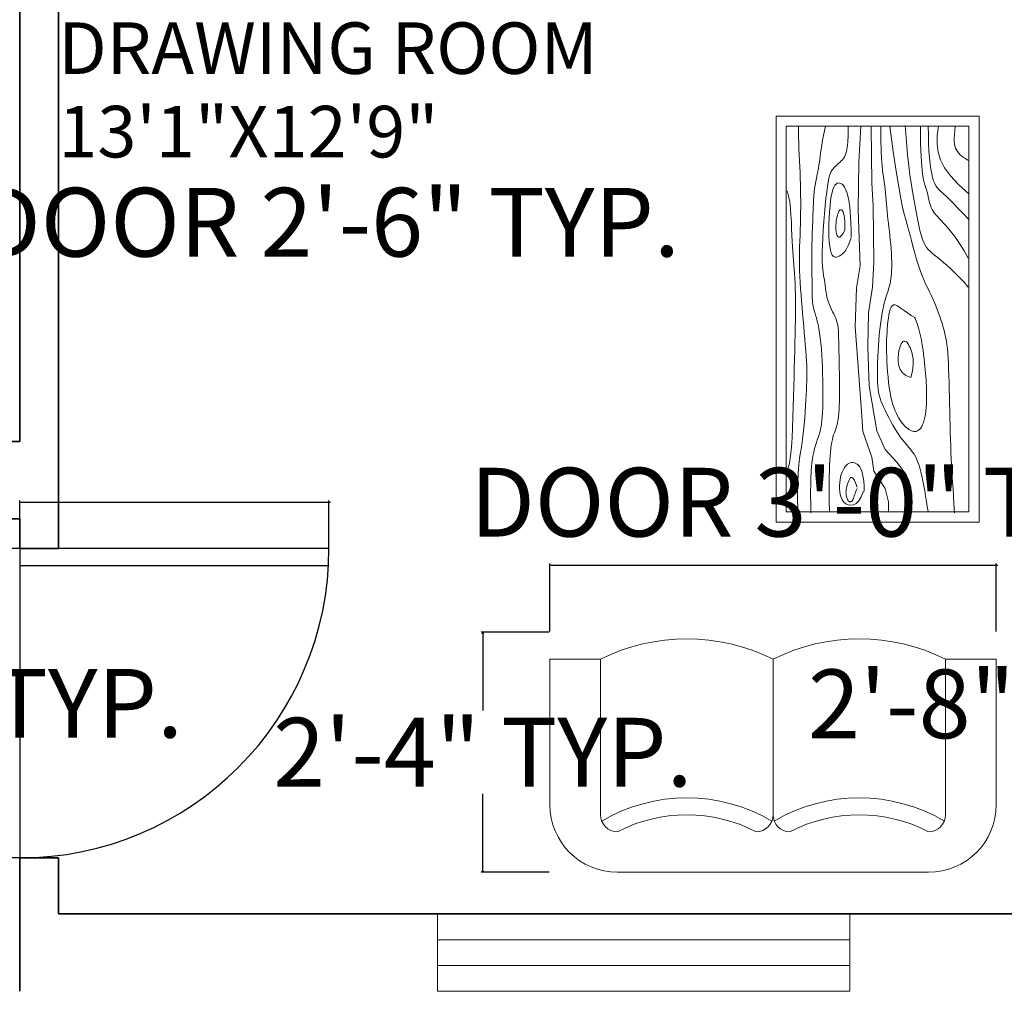
# Model space of a CAD drawing. Units: inches. Extents: x -11 to 443, y 65 to 743.
# Tile 3 of 10: x 162 to 276, y 212 to 325. Entities that reach past the tile are written whole.
import ezdxf

# ---------------------------------------------------------------- set-up
doc = ezdxf.new("R2010")
doc.units = ezdxf.units.IN
doc.header["$MEASUREMENT"] = 0
for name, color, linetype, lineweight in [('A-ANNO-DIMS', 2, 'Continuous', 18), ('A-AREA-IDEN', 2, 'Continuous', 18), ('A-DOOR', 4, 'Continuous', 25), ('A-GLAZ', 4, 'Continuous', 18), ('A-WALL', 7, 'Continuous', 35), ('Furniture', 7, 'Continuous', 15)]:
    doc.layers.add(name, color=color, linetype=linetype, lineweight=lineweight)
doc.styles.get("Standard").update_dxf_attribs({"font": 'italic8.shx'})
doc.dimstyles.get("Standard").update_dxf_attribs({"dimtxt": 8, "dimasz": 0.18, "dimexe": 0.18, "dimexo": 0.0625, "dimgap": 0.09, "dimtad": 0, "dimtih": 1, "dimtoh": 1, "dimzin": 0, "dimdsep": 46, "dimlunit": 3, "dimtxsty": 'Standard', "dimblk": 'CLOSEDBLANK', "dimcen": 0.09, "dimclrd": 6, "dimclre": 5, "dimclrt": 4, "dimadec": 0, "dimazin": 0, "dimtfac": 1, "dimtofl": 0, "dimtmove": 0, "dimatfit": 3, "dimfxl": 1, "dimtolj": 1, "dimtzin": 0, "dimarcsym": 0})

# ---------------------------------------------------------------- blocks, each defined once
blk = doc.blocks.new('DOOR-SWING-36')
for p, q in [((36, 36), (0, 36)), ((0, 36), (0, 0)), ((35.94, 34), (0, 34))]:
    blk.add_line(p, q)
blk.add_arc((0, 36), 36, 270, 0)
blk = doc.blocks.new('WIN-48x9')
for p, q in [((0, 48), (0, 0)), ((9, 48), (0, 48)), ((3, 0), (3, 48)), ((6, 0), (6, 48)), ((9, 0), (9, 48)), ((0, 0), (9, 0))]:
    blk.add_line(p, q)
blk = doc.blocks.new('LOVESEAT')
for p, q in [((0, 24.8, -27), (0, 7.87, -27)), ((0, 24.8, -27), (5.91, 24.8, -27)), ((5.91, 6.69, -27), (5.91, 24.8, -27)), ((25.98, 24.8, -27), (25.98, 6.69, -27)), ((25.98, 6.69, -27), (25.98, 24.8, -27)), ((46.06, 6.69, -27), (46.06, 24.8, -27)), ((46.06, 24.8, -27), (46.06, 6.69, -27)), ((46.06, 6.69, -27), (46.06, 24.8, -27)), ((51.97, 24.8, -27), (46.06, 24.8, -27)), ((51.97, 7.87, -27), (51.97, 24.8, -27)), ((7.87, 0, -27), (44.09, 0, -27))]:
    blk.add_line(p, q)
for centre, radius, start, end in [((15.94, 4.65, -27), 22.51, 63.519, 116.481), ((36.02, 4.65, -27), 22.51, 63.519, 116.481), ((15.94, -10.84, -27), 19.5, 59.4911, 120.5089), ((36.02, -10.84, -27), 19.5, 59.4911, 120.5089), ((7.87, 7.87, -27), 7.87, 180, 270), ((44.09, 7.87, -27), 7.87, 270, 0), ((7.87, 6.69, -27), 1.97, 180, 270), ((15.94, -10.84, -27), 17.53, 62.5861, 117.4139), ((24.02, 6.69, -27), 1.97, 270, 0), ((27.95, 6.69, -27), 1.97, 180, 270), ((36.02, -10.84, -27), 17.53, 62.5861, 117.4139), ((44.09, 6.69, -27), 1.97, 270, 0)]:
    blk.add_arc(centre, radius, start, end)
blk = doc.blocks.new('_ClosedBlank')
at = {"color": 0, "linetype": 'ByBlock', "lineweight": -2}
for p, q in [((-1, 0.167), (0, 0)), ((-1, 0.167), (-1, -0.167)), ((0, 0), (-1, -0.167))]:
    blk.add_line(p, q, dxfattribs=at)
blk = doc.blocks.new('*D20')
at = {"layer": 'A-ANNO-DIMS', "color": 5, "lineweight": -2, "transparency": 16777216}
for p, q in [((110.2, 296.98), (110.2, 301.6)), ((140.2, 296.98), (140.2, 301.6))]:
    blk.add_line(p, q, dxfattribs=at)
at = {"layer": 'A-ANNO-DIMS', "color": 6, "lineweight": -2, "transparency": 16777216}
for p, q in [((110.38, 301.42), (140.02, 301.42)), ((140.2, 301.42), (140.38, 301.42))]:
    blk.add_line(p, q, dxfattribs=at)
at = {"layer": 'Defpoints', "color": 0, "lineweight": 100, "transparency": 16777216}
for p in [(140.2, 301.42), (110.2, 296.92), (140.2, 296.92)]:
    blk.add_point(p, dxfattribs=at)
at = {"layer": 'A-ANNO-DIMS', "color": 6, "lineweight": -2, "transparency": 16777216, "xscale": 0.18, "yscale": 0.18, "zscale": 0.18, "rotation": 180}
blk.add_blockref('_ClosedBlank', (110.2, 301.42), dxfattribs=at)
at = {"layer": 'A-ANNO-DIMS', "color": 6, "lineweight": -2, "transparency": 16777216, "xscale": 0.18, "yscale": 0.18, "zscale": 0.18}
blk.add_blockref('_ClosedBlank', (140.2, 301.42), dxfattribs=at)
at = {"layer": 'A-ANNO-DIMS', "color": 4, "transparency": 16777216, "insert": (197.61, 301.42), "char_height": 8, "attachment_point": 5}
blk.add_mtext('\\A1;DOOR 2\'-6" TYP.', dxfattribs=at)
blk = doc.blocks.new('*D22')
at = {"layer": 'A-ANNO-DIMS', "color": 5, "lineweight": -2, "transparency": 16777216}
for p, q in [((161.71, 263.5), (161.71, 269.02)), ((197.71, 263.5), (197.71, 269.02))]:
    blk.add_line(p, q, dxfattribs=at)
at = {"layer": 'A-ANNO-DIMS', "color": 6, "lineweight": -2, "transparency": 16777216}
for p, q in [((161.89, 268.84), (197.53, 268.84)), ((197.71, 268.84), (197.89, 268.84))]:
    blk.add_line(p, q, dxfattribs=at)
at = {"layer": 'Defpoints', "color": 0, "lineweight": 100, "transparency": 16777216}
for p in [(197.71, 268.84), (161.71, 263.44), (197.71, 263.44)]:
    blk.add_point(p, dxfattribs=at)
at = {"layer": 'A-ANNO-DIMS', "color": 6, "lineweight": -2, "transparency": 16777216, "xscale": 0.18, "yscale": 0.18, "zscale": 0.18, "rotation": 180}
blk.add_blockref('_ClosedBlank', (161.71, 268.84), dxfattribs=at)
at = {"layer": 'A-ANNO-DIMS', "color": 6, "lineweight": -2, "transparency": 16777216, "xscale": 0.18, "yscale": 0.18, "zscale": 0.18}
blk.add_blockref('_ClosedBlank', (197.71, 268.84), dxfattribs=at)
at = {"layer": 'A-ANNO-DIMS', "color": 4, "transparency": 16777216, "insert": (255.12, 268.84), "char_height": 8, "attachment_point": 5}
blk.add_mtext('\\A1;DOOR 3\'-0" TYP.', dxfattribs=at)
blk = doc.blocks.new('*D23')
at = {"layer": 'A-ANNO-DIMS', "color": 5, "lineweight": -2, "transparency": 16777216}
for p, q in [((161.65, 263.44), (156.13, 263.44)), ((161.65, 227.44), (156.13, 227.44))]:
    blk.add_line(p, q, dxfattribs=at)
at = {"layer": 'A-ANNO-DIMS', "color": 6, "lineweight": -2, "transparency": 16777216}
for p, q in [((156.31, 263.26), (156.31, 250.29)), ((156.31, 227.62), (156.31, 240.59))]:
    blk.add_line(p, q, dxfattribs=at)
at = {"layer": 'Defpoints', "color": 0, "lineweight": 100, "transparency": 16777216}
for p in [(156.31, 263.44), (161.71, 263.44), (161.71, 227.44)]:
    blk.add_point(p, dxfattribs=at)
at = {"layer": 'A-ANNO-DIMS', "color": 6, "lineweight": -2, "transparency": 16777216, "xscale": 0.18, "yscale": 0.18, "zscale": 0.18}
for p, rotation in [((156.31, 263.44), 90), ((156.31, 227.44), 270)]:
    blk.add_blockref('_ClosedBlank', p, dxfattribs=dict(at, rotation=rotation))
at = {"layer": 'A-ANNO-DIMS', "color": 4, "transparency": 16777216, "insert": (156.31, 245.44), "char_height": 8, "attachment_point": 5}
blk.add_mtext('\\A1;3\'-0" TYP.', dxfattribs=at)
blk = doc.blocks.new('*D32')
at = {"layer": 'A-ANNO-DIMS', "color": 5, "lineweight": -2, "transparency": 16777216}
for p, q in [((223.42, 253.79), (223.42, 261.7)), ((275.39, 253.79), (275.39, 261.7))]:
    blk.add_line(p, q, dxfattribs=at)
at = {"layer": 'A-ANNO-DIMS', "color": 6, "lineweight": -2, "transparency": 16777216}
for p, q in [((223.6, 261.52), (275.21, 261.52)), ((275.39, 261.52), (275.57, 261.52))]:
    blk.add_line(p, q, dxfattribs=at)
at = {"layer": 'Defpoints', "color": 0, "lineweight": 100, "transparency": 16777216}
for p in [(275.39, 261.52), (223.42, 253.72), (275.39, 253.72)]:
    blk.add_point(p, dxfattribs=at)
at = {"layer": 'A-ANNO-DIMS', "color": 6, "lineweight": -2, "transparency": 16777216, "xscale": 0.18, "yscale": 0.18, "zscale": 0.18, "rotation": 180}
blk.add_blockref('_ClosedBlank', (223.42, 261.52), dxfattribs=at)
at = {"layer": 'A-ANNO-DIMS', "color": 6, "lineweight": -2, "transparency": 16777216, "xscale": 0.18, "yscale": 0.18, "zscale": 0.18}
blk.add_blockref('_ClosedBlank', (275.39, 261.52), dxfattribs=at)
at = {"layer": 'A-ANNO-DIMS', "color": 4, "transparency": 16777216, "insert": (349.75, 261.52), "char_height": 8, "attachment_point": 5}
blk.add_mtext('\\A1;LOVESEAT 4\'-4" TYP.', dxfattribs=at)
blk = doc.blocks.new('*D33')
at = {"layer": 'A-ANNO-DIMS', "color": 5, "lineweight": -2, "transparency": 16777216}
for p, q in [((223.36, 253.72), (215.44, 253.72)), ((223.36, 225.77), (215.44, 225.77))]:
    blk.add_line(p, q, dxfattribs=at)
at = {"layer": 'A-ANNO-DIMS', "color": 6, "lineweight": -2, "transparency": 16777216}
for p, q in [((215.62, 253.54), (215.62, 244.6)), ((215.62, 225.95), (215.62, 234.89))]:
    blk.add_line(p, q, dxfattribs=at)
at = {"layer": 'Defpoints', "color": 0, "lineweight": 100, "transparency": 16777216}
for p in [(215.62, 253.72), (223.42, 253.72), (223.42, 225.77)]:
    blk.add_point(p, dxfattribs=at)
at = {"layer": 'A-ANNO-DIMS', "color": 6, "lineweight": -2, "transparency": 16777216, "xscale": 0.18, "yscale": 0.18, "zscale": 0.18}
for p, rotation in [((215.62, 253.72), 90), ((215.62, 225.77), 270)]:
    blk.add_blockref('_ClosedBlank', p, dxfattribs=dict(at, rotation=rotation))
at = {"layer": 'A-ANNO-DIMS', "color": 4, "transparency": 16777216, "insert": (215.62, 239.75), "char_height": 8, "attachment_point": 5}
blk.add_mtext('\\A1;2\'-4" TYP.', dxfattribs=at)
blk = doc.blocks.new('*D35')
at = {"layer": 'A-ANNO-DIMS', "color": 5, "lineweight": -2, "transparency": 16777216}
for p, q in [((282.97, 261.39), (277.7, 261.39)), ((282.97, 229.35), (277.7, 229.35))]:
    blk.add_line(p, q, dxfattribs=at)
at = {"layer": 'A-ANNO-DIMS', "color": 6, "lineweight": -2, "transparency": 16777216}
for p, q in [((277.88, 261.21), (277.88, 250.22)), ((277.88, 229.53), (277.88, 240.52))]:
    blk.add_line(p, q, dxfattribs=at)
at = {"layer": 'Defpoints', "color": 0, "lineweight": 100, "transparency": 16777216}
for p in [(277.88, 261.39), (283.03, 261.39), (283.03, 229.35)]:
    blk.add_point(p, dxfattribs=at)
at = {"layer": 'A-ANNO-DIMS', "color": 6, "lineweight": -2, "transparency": 16777216, "xscale": 0.18, "yscale": 0.18, "zscale": 0.18}
for p, rotation in [((277.88, 261.39), 90), ((277.88, 229.35), 270)]:
    blk.add_blockref('_ClosedBlank', p, dxfattribs=dict(at, rotation=rotation))
at = {"layer": 'A-ANNO-DIMS', "color": 4, "transparency": 16777216, "insert": (277.88, 245.37), "char_height": 8, "attachment_point": 5}
blk.add_mtext('\\A1;2\'-8" TYP.', dxfattribs=at)

msp = doc.modelspace()

# ---------------------------------------------------------------- linework, layer by layer
at = {"layer": 'A-WALL'}
for p, q in [((161.709, 275.92), (161.709, 373.92)), ((166.209, 263.442), (166.209, 373.92)), ((140.201, 275.92), (161.709, 275.92)), ((140.201, 266.92), (161.709, 266.92)), ((161.709, 263.442), (161.709, 266.92)), ((161.709, 263.442), (166.209, 263.442)), ((161.709, 211.92), (161.709, 227.442)), ((161.709, 227.442), (166.209, 227.442)), ((166.209, 220.92), (166.209, 227.442)), ((166.209, 220.92), (323.209, 220.92))]:
    msp.add_line(p, q, dxfattribs=at)
at = {"layer": 'Furniture'}
for p, q in [((249.755, 266.524), (249.755, 313.768)), ((249.755, 313.768), (273.377, 313.768)), ((273.377, 313.768), (273.377, 266.524)), ((250.936, 267.705), (250.936, 312.587)), ((250.936, 312.587), (272.196, 312.587)), ((252.347, 312.524), (252.353, 311.905)), ((252.353, 311.905), (252.367, 311.265)), ((255.496, 312.605), (255.31, 311.718)), ((258.161, 312.524), (258.146, 311.54)), ((259.614, 312.605), (259.372, 308.404)), ((260.826, 312.524), (260.906, 305.98)), ((261.956, 312.524), (261.967, 311.013)), ((263.006, 312.605), (263.399, 309.671)), ((264.782, 312.685), (264.93, 310.824)), ((266.559, 312.524), (266.578, 310.594)), ((267.474, 312.632), (267.483, 311.568)), ((268.658, 312.605), (268.522, 311.512)), ((270.543, 312.067), (270.507, 311.601)), ((270.596, 312.605), (270.543, 312.067)), ((272.196, 312.587), (272.196, 267.705)), ((252.367, 311.265), (252.39, 310.606)), ((252.39, 310.606), (252.417, 309.934)), ((255.168, 310.983), (255.062, 310.374)), ((255.31, 311.718), (255.168, 310.983)), ((258.105, 310.754), (258.04, 310.138)), ((258.146, 311.54), (258.105, 310.754)), ((261.967, 311.013), (261.996, 309.787)), ((264.93, 310.824), (265.071, 309.271)), ((267.483, 311.568), (267.51, 310.597)), ((267.51, 310.597), (267.554, 309.716)), ((268.522, 311.512), (268.498, 310.516)), ((270.507, 311.601), (270.49, 311.198)), ((270.49, 311.198), (270.492, 310.85)), ((270.492, 310.85), (270.517, 310.548)), ((252.417, 309.934), (252.448, 309.253)), ((254.985, 309.868), (254.928, 309.442)), ((255.062, 310.374), (254.985, 309.868)), ((257.954, 309.667), (257.851, 309.313)), ((258.04, 310.138), (257.954, 309.667)), ((261.996, 309.787), (262.04, 308.803)), ((263.399, 309.671), (263.735, 307.353)), ((266.578, 310.594), (266.632, 309.07)), ((267.554, 309.716), (267.612, 308.925)), ((268.498, 310.516), (268.611, 309.581)), ((268.611, 309.581), (268.89, 308.676)), ((270.517, 310.548), (270.565, 310.284)), ((270.565, 310.284), (270.638, 310.05)), ((270.638, 310.05), (270.737, 309.838)), ((270.737, 309.838), (270.864, 309.64)), ((270.864, 309.64), (271.016, 309.454)), ((271.016, 309.454), (271.187, 309.281)), ((252.448, 309.253), (252.481, 308.567)), ((252.481, 308.567), (252.513, 307.881)), ((254.797, 308.404), (254.74, 308.063)), ((254.842, 308.733), (254.797, 308.404)), ((254.883, 309.071), (254.842, 308.733)), ((254.928, 309.442), (254.883, 309.071)), ((257.197, 308.416), (257.056, 308.288)), ((257.337, 308.55), (257.197, 308.416)), ((257.475, 308.693), (257.337, 308.55)), ((257.608, 308.853), (257.475, 308.693)), ((257.735, 309.05), (257.608, 308.853)), ((257.851, 309.313), (257.735, 309.05)), ((259.372, 308.404), (259.291, 302.829)), ((262.04, 308.803), (262.096, 308.02)), ((265.071, 309.271), (265.206, 307.98)), ((266.632, 309.07), (266.712, 307.892)), ((267.612, 308.925), (267.686, 308.22)), ((268.89, 308.676), (269.362, 307.768)), ((271.187, 309.281), (271.376, 309.118)), ((271.376, 309.118), (271.576, 308.966)), ((271.576, 308.966), (271.785, 308.824)), ((271.785, 308.824), (271.998, 308.69)), ((271.998, 308.69), (272.211, 308.565)), ((252.513, 307.881), (252.542, 307.199)), ((252.542, 307.199), (252.568, 306.523)), ((254.602, 307.34), (254.526, 306.96)), ((254.674, 307.708), (254.602, 307.34)), ((254.74, 308.063), (254.674, 307.708)), ((256.182, 307.327), (256.084, 307.114)), ((256.286, 307.501), (256.182, 307.327)), ((256.398, 307.65), (256.286, 307.501)), ((256.518, 307.786), (256.398, 307.65)), ((256.646, 307.916), (256.518, 307.786)), ((256.779, 308.041), (256.646, 307.916)), ((256.916, 308.164), (256.779, 308.041)), ((257.056, 308.288), (256.916, 308.164)), ((262.096, 308.02), (262.158, 307.396)), ((262.158, 307.396), (262.223, 306.889)), ((263.735, 307.353), (264.024, 305.557)), ((265.206, 307.98), (265.336, 306.908)), ((266.712, 307.892), (266.812, 307.005)), ((267.686, 308.22), (267.772, 307.6)), ((267.772, 307.6), (267.87, 307.063)), ((269.362, 307.768), (270.055, 306.822)), ((252.568, 306.523), (252.589, 305.855)), ((254.375, 306.166), (254.306, 305.754)), ((254.449, 306.568), (254.375, 306.166)), ((254.526, 306.96), (254.449, 306.568)), ((255.815, 306.091), (255.73, 305.574)), ((255.902, 306.511), (255.815, 306.091)), ((255.991, 306.847), (255.902, 306.511)), ((256.084, 307.114), (255.991, 306.847)), ((262.223, 306.889), (262.287, 306.458)), ((262.287, 306.458), (262.346, 306.061)), ((262.346, 306.061), (262.398, 305.663)), ((265.336, 306.908), (265.461, 306.01)), ((266.812, 307.005), (266.923, 306.351)), ((266.923, 306.351), (267.038, 305.872)), ((267.87, 307.063), (267.978, 306.606)), ((267.978, 306.606), (268.097, 306.227)), ((268.097, 306.227), (268.224, 305.916)), ((270.055, 306.822), (270.995, 305.806)), ((251.055, 305.091), (251.215, 304.472)), ((252.589, 305.855), (252.605, 305.191)), ((252.605, 305.191), (252.616, 304.532)), ((254.195, 304.906), (254.154, 304.474)), ((254.245, 305.334), (254.195, 304.906)), ((254.306, 305.754), (254.245, 305.334)), ((255.644, 304.943), (255.558, 304.193)), ((255.73, 305.574), (255.644, 304.943)), ((256.275, 304.886), (256.183, 304.453)), ((256.377, 305.237), (256.275, 304.886)), ((256.487, 305.514), (256.377, 305.237)), ((256.606, 305.722), (256.487, 305.514)), ((256.732, 305.867), (256.606, 305.722)), ((256.865, 305.955), (256.732, 305.867)), ((257.004, 305.994), (256.865, 305.955)), ((257.147, 305.986), (257.004, 305.994)), ((257.293, 305.934), (257.147, 305.986)), ((257.439, 305.835), (257.293, 305.934)), ((257.583, 305.688), (257.439, 305.835)), ((257.722, 305.492), (257.583, 305.688)), ((257.854, 305.247), (257.722, 305.492)), ((257.977, 304.95), (257.854, 305.247)), ((258.087, 304.6), (257.977, 304.95)), ((260.906, 305.98), (261.068, 303.314)), ((262.398, 305.663), (262.442, 305.258)), ((262.442, 305.258), (262.482, 304.846)), ((264.024, 305.557), (264.272, 304.19)), ((265.461, 306.01), (265.583, 305.241)), ((265.583, 305.241), (265.702, 304.557)), ((267.038, 305.872), (267.15, 305.512)), ((267.15, 305.512), (267.252, 305.213)), ((267.252, 305.213), (267.337, 304.927)), ((267.337, 304.927), (267.408, 304.646)), ((268.224, 305.916), (268.36, 305.66)), ((268.36, 305.66), (268.504, 305.449)), ((268.504, 305.449), (268.656, 305.271)), ((268.656, 305.271), (268.816, 305.115)), ((268.816, 305.115), (268.982, 304.969)), ((268.982, 304.969), (269.156, 304.822)), ((270.995, 305.806), (272.211, 304.688)), ((251.215, 304.472), (251.337, 303.779)), ((251.337, 303.779), (251.426, 303.032)), ((252.616, 304.532), (252.621, 303.874)), ((252.621, 303.874), (252.621, 303.218)), ((254.122, 304.038), (254.097, 303.602)), ((254.154, 304.474), (254.122, 304.038)), ((255.558, 304.193), (255.474, 303.347)), ((256.102, 303.933), (256.032, 303.326)), ((256.183, 304.453), (256.102, 303.933)), ((258.183, 304.197), (258.087, 304.6)), ((258.265, 303.737), (258.183, 304.197)), ((258.334, 303.22), (258.265, 303.737)), ((262.482, 304.846), (262.518, 304.427)), ((262.518, 304.427), (262.553, 304)), ((262.553, 304), (262.589, 303.567)), ((264.272, 304.19), (264.487, 303.159)), ((265.702, 304.557), (265.818, 303.913)), ((265.818, 303.913), (265.934, 303.274)), ((267.408, 304.646), (267.47, 304.371)), ((267.47, 304.371), (267.528, 304.103)), ((267.528, 304.103), (267.587, 303.844)), ((267.587, 303.844), (267.65, 303.594)), ((269.156, 304.822), (269.338, 304.661)), ((269.338, 304.661), (269.544, 304.471)), ((269.544, 304.471), (269.789, 304.233)), ((269.789, 304.233), (270.089, 303.93)), ((270.089, 303.93), (270.463, 303.545)), ((251.426, 303.032), (251.489, 302.253)), ((252.621, 303.218), (252.615, 302.56)), ((254.059, 302.738), (254.044, 302.315)), ((254.076, 303.168), (254.059, 302.738)), ((254.097, 303.602), (254.076, 303.168)), ((255.474, 303.347), (255.393, 302.435)), ((255.975, 302.65), (255.933, 301.932)), ((256.032, 303.326), (255.975, 302.65)), ((257.059, 302.692), (257.002, 302.568)), ((257.12, 302.786), (257.059, 302.692)), ((257.183, 302.848), (257.12, 302.786)), ((257.25, 302.877), (257.183, 302.848)), ((257.32, 302.871), (257.25, 302.877)), ((257.394, 302.829), (257.32, 302.871)), ((257.471, 302.749), (257.394, 302.829)), ((257.547, 302.622), (257.471, 302.749)), ((257.619, 302.443), (257.547, 302.622)), ((258.389, 302.642), (258.334, 303.22)), ((258.431, 302.001), (258.389, 302.642)), ((259.291, 302.829), (259.534, 296.366)), ((261.068, 303.314), (261.149, 296.77)), ((262.589, 303.567), (262.627, 303.127)), ((262.627, 303.127), (262.669, 302.681)), ((262.669, 302.681), (262.718, 302.229)), ((264.487, 303.159), (264.678, 302.372)), ((265.934, 303.274), (266.049, 302.639)), ((266.049, 302.639), (266.166, 302.017)), ((267.65, 303.594), (267.723, 303.354)), ((267.723, 303.354), (267.81, 303.126)), ((267.81, 303.126), (267.915, 302.909)), ((267.915, 302.909), (268.04, 302.7)), ((268.04, 302.7), (268.184, 302.495)), ((270.463, 303.545), (270.925, 303.061)), ((270.925, 303.061), (271.493, 302.46)), ((251.489, 302.253), (251.534, 301.462)), ((251.534, 301.462), (251.566, 300.681)), ((252.603, 301.9), (252.585, 301.237)), ((252.615, 302.56), (252.603, 301.9)), ((254.014, 301.496), (253.998, 301.095)), ((254.029, 301.9), (254.014, 301.496)), ((254.044, 302.315), (254.029, 301.9)), ((255.318, 301.49), (255.252, 300.542)), ((255.393, 302.435), (255.318, 301.49)), ((255.933, 301.932), (255.907, 301.199)), ((256.765, 301.57), (256.735, 301.32)), ((256.803, 301.809), (256.765, 301.57)), ((256.847, 302.033), (256.803, 301.809)), ((256.896, 302.237), (256.847, 302.033)), ((256.948, 302.416), (256.896, 302.237)), ((257.002, 302.568), (256.948, 302.416)), ((257.682, 302.203), (257.619, 302.443)), ((257.731, 301.895), (257.682, 302.203)), ((257.763, 301.512), (257.731, 301.895)), ((257.773, 301.045), (257.763, 301.512)), ((258.461, 301.295), (258.431, 302.001)), ((262.718, 302.229), (262.771, 301.769)), ((262.771, 301.769), (262.827, 301.303)), ((264.678, 302.372), (264.852, 301.734)), ((264.852, 301.734), (265.018, 301.153)), ((266.166, 302.017), (266.284, 301.418)), ((268.184, 302.495), (268.347, 302.289)), ((268.347, 302.289), (268.529, 302.077)), ((268.529, 302.077), (268.732, 301.855)), ((268.732, 301.855), (268.954, 301.618)), ((268.954, 301.618), (269.196, 301.362)), ((271.493, 302.46), (272.184, 301.725)), ((251.566, 300.681), (251.593, 299.929)), ((252.563, 300.57), (252.54, 299.899)), ((252.585, 301.237), (252.563, 300.57)), ((253.981, 300.691), (253.966, 300.276)), ((253.998, 301.095), (253.981, 300.691)), ((255.252, 300.542), (255.198, 299.623)), ((255.907, 301.199), (255.898, 300.474)), ((255.898, 300.474), (255.909, 299.785)), ((256.716, 301.064), (256.71, 300.807)), ((256.71, 300.807), (256.717, 300.555)), ((256.735, 301.32), (256.716, 301.064)), ((256.717, 300.555), (256.741, 300.312)), ((256.741, 300.312), (256.783, 300.084)), ((257.532, 300.082), (257.757, 300.487)), ((257.757, 300.487), (257.773, 301.045)), ((258.478, 300.522), (258.461, 301.295)), ((258.484, 299.679), (258.478, 300.522)), ((262.827, 301.303), (262.885, 300.828)), ((262.885, 300.828), (262.942, 300.346)), ((262.942, 300.346), (262.999, 299.854)), ((265.018, 301.153), (265.182, 300.554)), ((265.182, 300.554), (265.346, 299.928)), ((266.284, 301.418), (266.406, 300.85)), ((266.406, 300.85), (266.532, 300.322)), ((266.532, 300.322), (266.663, 299.844)), ((269.196, 301.362), (269.459, 301.08)), ((269.459, 301.08), (269.745, 300.76)), ((269.745, 300.76), (270.058, 300.388)), ((270.058, 300.388), (270.401, 299.95)), ((251.593, 299.929), (251.621, 299.228)), ((251.621, 299.228), (251.654, 298.592)), ((252.517, 299.224), (252.498, 298.546)), ((252.54, 299.899), (252.517, 299.224)), ((253.939, 299.384), (253.929, 298.892)), ((253.951, 299.843), (253.939, 299.384)), ((253.966, 300.276), (253.951, 299.843)), ((255.198, 299.623), (255.157, 298.764)), ((255.909, 299.785), (255.94, 299.157)), ((255.94, 299.157), (255.994, 298.615)), ((256.783, 300.084), (256.846, 299.89)), ((256.846, 299.89), (256.931, 299.748)), ((256.931, 299.748), (257.04, 299.677)), ((257.04, 299.677), (257.175, 299.696)), ((257.175, 299.696), (257.338, 299.825)), ((257.338, 299.825), (257.532, 300.082)), ((258.201, 298.792), (258.352, 299.17)), ((258.352, 299.17), (258.484, 299.598)), ((262.999, 299.854), (263.052, 299.354)), ((263.052, 299.354), (263.1, 298.844)), ((265.346, 299.928), (265.511, 299.285)), ((265.511, 299.285), (265.68, 298.636)), ((266.663, 299.844), (266.801, 299.423)), ((266.801, 299.423), (266.947, 299.065)), ((270.401, 299.95), (270.776, 299.431)), ((270.776, 299.431), (271.187, 298.819)), ((251.654, 298.592), (251.694, 298.013)), ((251.694, 298.013), (251.737, 297.477)), ((252.498, 298.546), (252.484, 297.864)), ((253.922, 298.359), (253.919, 297.782)), ((253.929, 298.892), (253.922, 298.359)), ((255.133, 297.996), (255.127, 297.342)), ((255.157, 298.764), (255.133, 297.996)), ((255.994, 298.615), (256.072, 298.18)), ((256.072, 298.18), (256.171, 297.847)), ((257.67, 297.943), (257.857, 298.181)), ((257.857, 298.181), (258.035, 298.463)), ((258.035, 298.463), (258.201, 298.792)), ((263.1, 298.844), (263.142, 298.325)), ((263.142, 298.325), (263.176, 297.802)), ((265.68, 298.636), (265.851, 297.99)), ((265.851, 297.99), (266.027, 297.356)), ((266.947, 299.065), (267.104, 298.762)), ((267.104, 298.762), (267.277, 298.5)), ((267.277, 298.5), (267.469, 298.266)), ((267.469, 298.266), (267.684, 298.047)), ((267.684, 298.047), (267.927, 297.831)), ((271.187, 298.819), (271.637, 298.098)), ((271.637, 298.098), (272.13, 297.255)), ((251.737, 297.477), (251.782, 296.968)), ((251.782, 296.968), (251.827, 296.473)), ((252.484, 297.864), (252.478, 297.178)), ((252.478, 297.178), (252.482, 296.488)), ((253.919, 297.782), (253.918, 297.173)), ((253.918, 297.173), (253.921, 296.545)), ((255.127, 297.342), (255.137, 296.793)), ((256.171, 297.847), (256.289, 297.608)), ((256.289, 297.608), (256.425, 297.452)), ((256.425, 297.452), (256.576, 297.37)), ((256.576, 297.37), (256.74, 297.352)), ((256.74, 297.352), (256.915, 297.389)), ((256.915, 297.389), (257.098, 297.471)), ((257.098, 297.471), (257.287, 297.59)), ((257.287, 297.59), (257.479, 297.746)), ((257.479, 297.746), (257.67, 297.943)), ((263.176, 297.802), (263.201, 297.28)), ((263.201, 297.28), (263.214, 296.765)), ((266.027, 297.356), (266.209, 296.744)), ((267.927, 297.831), (268.201, 297.605)), ((268.201, 297.605), (268.51, 297.356)), ((268.51, 297.356), (268.857, 297.073)), ((268.857, 297.073), (269.24, 296.751)), ((251.827, 296.473), (251.87, 295.978)), ((251.87, 295.978), (251.91, 295.467)), ((252.482, 296.488), (252.498, 295.794)), ((252.498, 295.794), (252.525, 295.096)), ((253.921, 296.545), (253.925, 295.915)), ((253.925, 295.915), (253.931, 295.298)), ((255.137, 296.793), (255.16, 296.331)), ((255.16, 296.331), (255.194, 295.939)), ((255.194, 295.939), (255.235, 295.598)), ((259.534, 296.366), (259.13, 293.781)), ((261.149, 296.77), (260.987, 293.862)), ((263.202, 295.782), (263.173, 295.325)), ((263.215, 296.264), (263.202, 295.782)), ((263.214, 296.765), (263.215, 296.264)), ((266.209, 296.744), (266.397, 296.165)), ((266.397, 296.165), (266.592, 295.624)), ((269.24, 296.751), (269.657, 296.387)), ((269.657, 296.387), (270.103, 295.98)), ((270.103, 295.98), (270.577, 295.527)), ((251.91, 295.467), (251.944, 294.926)), ((251.944, 294.926), (251.97, 294.344)), ((252.525, 295.096), (252.563, 294.393)), ((253.931, 295.298), (253.937, 294.709)), ((253.937, 294.709), (253.943, 294.162)), ((255.235, 295.598), (255.281, 295.292)), ((255.281, 295.292), (255.328, 295.002)), ((255.328, 295.002), (255.375, 294.71)), ((255.375, 294.71), (255.419, 294.404)), ((263.127, 294.899), (263.062, 294.507)), ((263.173, 295.325), (263.127, 294.899)), ((266.592, 295.624), (266.793, 295.119)), ((266.793, 295.119), (266.997, 294.644)), ((266.997, 294.644), (267.203, 294.194)), ((270.577, 295.527), (271.074, 295.024)), ((271.074, 295.024), (271.593, 294.47)), ((251.97, 294.344), (251.99, 293.719)), ((251.99, 293.719), (252.002, 293.053)), ((252.563, 294.393), (252.608, 293.685)), ((252.608, 293.685), (252.66, 292.972)), ((253.943, 294.162), (253.949, 293.674)), ((253.949, 293.674), (253.954, 293.254)), ((255.419, 294.404), (255.462, 294.083)), ((255.462, 294.083), (255.507, 293.752)), ((255.507, 293.752), (255.555, 293.416)), ((255.555, 293.416), (255.611, 293.08)), ((259.13, 293.781), (258.968, 289.257)), ((260.987, 293.862), (260.503, 290.873)), ((262.787, 293.456), (262.678, 293.118)), ((262.889, 293.795), (262.787, 293.456)), ((262.982, 294.142), (262.889, 293.795)), ((263.062, 294.507), (262.982, 294.142)), ((267.203, 294.194), (267.408, 293.761)), ((267.408, 293.761), (267.61, 293.341)), ((271.593, 294.47), (272.13, 293.862)), ((252.002, 293.053), (252.009, 292.349)), ((252.009, 292.349), (252.01, 291.607)), ((252.66, 292.972), (252.718, 292.252)), ((253.954, 293.254), (253.959, 292.896)), ((253.959, 292.896), (253.967, 292.589)), ((253.967, 292.589), (253.981, 292.32)), ((253.981, 292.32), (254.001, 292.08)), ((255.611, 293.08), (255.676, 292.747)), ((255.676, 292.747), (255.754, 292.423)), ((255.754, 292.423), (255.846, 292.112)), ((262.455, 292.401), (262.346, 292.004)), ((262.567, 292.769), (262.455, 292.401)), ((262.678, 293.118), (262.567, 292.769)), ((267.61, 293.341), (267.808, 292.928)), ((267.808, 292.928), (267.999, 292.516)), ((267.999, 292.516), (268.181, 292.1)), ((252.01, 291.607), (252.006, 290.83)), ((252.718, 292.252), (252.78, 291.526)), ((252.78, 291.526), (252.845, 290.792)), ((254.001, 292.08), (254.03, 291.856)), ((254.03, 291.856), (254.07, 291.637)), ((254.07, 291.637), (254.124, 291.412)), ((254.124, 291.412), (254.191, 291.17)), ((254.191, 291.17), (254.271, 290.905)), ((255.846, 292.112), (255.955, 291.817)), ((255.955, 291.817), (256.077, 291.537)), ((256.077, 291.537), (256.207, 291.268)), ((256.207, 291.268), (256.339, 291.008)), ((262.244, 291.571), (262.147, 291.104)), ((262.346, 292.004), (262.244, 291.571)), ((262.965, 290.992), (263.052, 291.294)), ((263.052, 291.294), (263.158, 291.538)), ((263.158, 291.538), (263.283, 291.711)), ((263.283, 291.711), (263.43, 291.802)), ((263.43, 291.802), (263.602, 291.802)), ((263.602, 291.802), (263.805, 291.722)), ((263.805, 291.722), (264.044, 291.574)), ((264.044, 291.574), (264.325, 291.373)), ((264.325, 291.373), (264.655, 291.132)), ((264.655, 291.132), (265.039, 290.865)), ((268.181, 292.1), (268.354, 291.682)), ((268.354, 291.682), (268.518, 291.265)), ((268.518, 291.265), (268.671, 290.853)), ((251.997, 290.019), (251.984, 289.176)), ((252.006, 290.83), (251.997, 290.019)), ((252.845, 290.792), (252.911, 290.053)), ((252.911, 290.053), (252.977, 289.313)), ((254.271, 290.905), (254.359, 290.611)), ((254.359, 290.611), (254.453, 290.284)), ((254.453, 290.284), (254.55, 289.918)), ((256.339, 291.008), (256.47, 290.752)), ((256.47, 290.752), (256.594, 290.499)), ((256.594, 290.499), (256.706, 290.244)), ((256.706, 290.244), (256.802, 289.984)), ((256.802, 289.984), (256.877, 289.717)), ((260.503, 290.873), (260.422, 286.914)), ((261.975, 290.072), (261.899, 289.513)), ((262.057, 290.603), (261.975, 290.072)), ((262.147, 291.104), (262.057, 290.603)), ((262.78, 289.859), (262.831, 290.263)), ((262.831, 290.263), (262.891, 290.645)), ((262.891, 290.645), (262.965, 290.992)), ((265.039, 290.865), (265.483, 290.585)), ((265.483, 290.585), (265.993, 290.307)), ((265.913, 290.307), (266.161, 289.644)), ((268.671, 290.853), (268.815, 290.448)), ((268.815, 290.448), (268.949, 290.054)), ((268.949, 290.054), (269.071, 289.674)), ((251.984, 289.176), (251.967, 288.303)), ((252.977, 289.313), (253.041, 288.581)), ((254.55, 289.918), (254.646, 289.507)), ((254.646, 289.507), (254.738, 289.046)), ((254.738, 289.046), (254.823, 288.53)), ((256.877, 289.717), (256.934, 289.435)), ((256.934, 289.435), (256.976, 289.131)), ((256.976, 289.131), (257.005, 288.798)), ((258.968, 289.257), (259.372, 283.602)), ((261.83, 288.929), (261.768, 288.322)), ((261.899, 289.513), (261.83, 288.929)), ((262.667, 288.616), (262.699, 289.032)), ((262.699, 289.032), (262.737, 289.446)), ((262.737, 289.446), (262.78, 289.859)), ((266.161, 289.644), (266.366, 288.989)), ((266.366, 288.989), (266.533, 288.347)), ((269.071, 289.674), (269.183, 289.311)), ((269.183, 289.311), (269.283, 288.966)), ((269.283, 288.966), (269.373, 288.63)), ((251.967, 288.303), (251.947, 287.396)), ((253.041, 288.581), (253.103, 287.864)), ((253.103, 287.864), (253.159, 287.169)), ((254.823, 288.53), (254.899, 287.956)), ((254.899, 287.956), (254.965, 287.331)), ((257.005, 288.798), (257.025, 288.429)), ((257.025, 288.429), (257.038, 288.017)), ((257.038, 288.017), (257.048, 287.555)), ((261.714, 287.695), (261.667, 287.052)), ((261.768, 288.322), (261.714, 287.695)), ((262.611, 287.302), (262.622, 287.756)), ((262.622, 287.756), (262.641, 288.192)), ((262.641, 288.192), (262.667, 288.616)), ((266.533, 288.347), (266.667, 287.723)), ((266.667, 287.723), (266.773, 287.123)), ((269.373, 288.63), (269.453, 288.292)), ((269.453, 288.292), (269.524, 287.941)), ((269.524, 287.941), (269.587, 287.566)), ((251.947, 287.396), (251.924, 286.454)), ((253.159, 287.169), (253.21, 286.505)), ((254.965, 287.331), (255.022, 286.666)), ((255.022, 286.666), (255.071, 285.969)), ((257.048, 287.555), (257.057, 287.036)), ((257.057, 287.036), (257.069, 286.455)), ((260.422, 286.914), (260.583, 282.39)), ((261.667, 287.052), (261.628, 286.4)), ((262.608, 286.825), (262.611, 287.302)), ((262.614, 286.321), (262.608, 286.825)), ((264.144, 286.808), (264.062, 286.477)), ((264.233, 287.073), (264.144, 286.808)), ((264.327, 287.277), (264.233, 287.073)), ((264.425, 287.425), (264.327, 287.277)), ((264.525, 287.523), (264.425, 287.425)), ((264.625, 287.574), (264.525, 287.523)), ((264.725, 287.585), (264.625, 287.574)), ((264.823, 287.561), (264.725, 287.585)), ((264.917, 287.505), (264.823, 287.561)), ((265.007, 287.421), (264.917, 287.505)), ((265.095, 287.31), (265.007, 287.421)), ((265.18, 287.174), (265.095, 287.31)), ((265.263, 287.013), (265.18, 287.174)), ((265.344, 286.83), (265.263, 287.013)), ((265.424, 286.626), (265.344, 286.83)), ((265.502, 286.403), (265.424, 286.626)), ((266.773, 287.123), (266.858, 286.55)), ((266.858, 286.55), (266.926, 286.01)), ((269.587, 287.566), (269.643, 287.156)), ((269.643, 287.156), (269.692, 286.7)), ((269.692, 286.7), (269.735, 286.187)), ((251.898, 285.475), (251.871, 284.455)), ((251.924, 286.454), (251.898, 285.475)), ((253.21, 286.505), (253.254, 285.879)), ((253.254, 285.879), (253.289, 285.299)), ((255.071, 285.969), (255.111, 285.25)), ((257.069, 286.455), (257.081, 285.825)), ((257.081, 285.825), (257.095, 285.157)), ((261.598, 285.75), (261.576, 285.11)), ((261.628, 286.4), (261.598, 285.75)), ((262.629, 285.783), (262.614, 286.321)), ((262.654, 285.211), (262.629, 285.783)), ((263.991, 286.079), (263.949, 285.635)), ((263.949, 285.635), (263.956, 285.168)), ((264.062, 286.477), (263.991, 286.079)), ((265.579, 286.16), (265.502, 286.403)), ((265.647, 285.893), (265.579, 286.16)), ((265.698, 285.594), (265.647, 285.893)), ((265.725, 285.255), (265.698, 285.594)), ((266.926, 286.01), (266.982, 285.507)), ((266.982, 285.507), (267.033, 285.045)), ((269.735, 286.187), (269.773, 285.609)), ((269.773, 285.609), (269.806, 284.971)), ((251.871, 284.455), (251.842, 283.393)), ((253.289, 285.299), (253.315, 284.767)), ((253.315, 284.767), (253.331, 284.275)), ((253.331, 284.275), (253.338, 283.806)), ((255.111, 285.25), (255.143, 284.52)), ((255.143, 284.52), (255.168, 283.788)), ((257.095, 285.157), (257.108, 284.467)), ((257.108, 284.467), (257.12, 283.768)), ((261.563, 284.491), (261.559, 283.901)), ((261.576, 285.11), (261.563, 284.491)), ((262.69, 284.612), (262.654, 285.211)), ((262.736, 283.997), (262.69, 284.612)), ((263.956, 285.168), (264.031, 284.704)), ((264.031, 284.704), (264.196, 284.266)), ((264.196, 284.266), (264.47, 283.88)), ((265.579, 283.929), (265.673, 284.43)), ((265.673, 284.43), (265.719, 284.869)), ((265.719, 284.869), (265.725, 285.255)), ((267.033, 285.045), (267.077, 284.617)), ((267.077, 284.617), (267.117, 284.216)), ((269.806, 284.971), (269.836, 284.28)), ((269.836, 284.28), (269.862, 283.545)), ((251.842, 283.393), (251.812, 282.286)), ((253.336, 283.348), (253.328, 282.885)), ((253.338, 283.806), (253.336, 283.348)), ((255.168, 283.788), (255.187, 283.064)), ((257.12, 283.768), (257.129, 283.075)), ((259.372, 283.602), (259.695, 279.401)), ((261.559, 283.901), (261.564, 283.35)), ((261.564, 283.35), (261.579, 282.848)), ((262.792, 283.378), (262.736, 283.997)), ((262.859, 282.766), (262.792, 283.378)), ((264.47, 283.88), (264.874, 283.57)), ((264.874, 283.57), (265.428, 283.36)), ((265.428, 283.36), (265.579, 283.929)), ((267.117, 284.216), (267.152, 283.834)), ((267.152, 283.834), (267.181, 283.462)), ((267.181, 283.462), (267.207, 283.094)), ((267.207, 283.094), (267.228, 282.722)), ((269.862, 283.545), (269.886, 282.773)), ((251.812, 282.286), (251.782, 281.131)), ((253.312, 282.404), (253.29, 281.889)), ((253.328, 282.885), (253.312, 282.404)), ((255.187, 283.064), (255.199, 282.356)), ((255.199, 282.356), (255.204, 281.672)), ((257.129, 283.075), (257.136, 282.4)), ((257.136, 282.4), (257.138, 281.758)), ((260.583, 282.39), (261.472, 277.139)), ((261.579, 282.848), (261.605, 282.401)), ((261.605, 282.401), (261.643, 282)), ((261.643, 282), (261.695, 281.634)), ((262.937, 282.173), (262.859, 282.766)), ((263.027, 281.608), (262.937, 282.173)), ((267.228, 282.722), (267.245, 282.337)), ((267.245, 282.337), (267.258, 281.934)), ((269.886, 282.773), (269.909, 281.973)), ((269.909, 281.973), (269.93, 281.151)), ((251.782, 281.131), (251.751, 279.933)), ((253.262, 281.327), (253.229, 280.707)), ((253.29, 281.889), (253.262, 281.327)), ((255.203, 281.016), (255.195, 280.394)), ((255.204, 281.672), (255.203, 281.016)), ((257.136, 281.16), (257.127, 280.607)), ((257.138, 281.758), (257.136, 281.16)), ((261.695, 281.634), (261.764, 281.291)), ((261.764, 281.291), (261.852, 280.961)), ((261.852, 280.961), (261.962, 280.631)), ((263.127, 281.084), (263.027, 281.608)), ((263.238, 280.61), (263.127, 281.084)), ((267.258, 281.934), (267.266, 281.517)), ((267.268, 281.092), (267.262, 280.665)), ((267.266, 281.517), (267.268, 281.092)), ((269.93, 281.151), (269.95, 280.317)), ((251.751, 279.933), (251.715, 278.714)), ((253.191, 280.041), (253.146, 279.341)), ((253.229, 280.707), (253.191, 280.041)), ((255.18, 279.811), (255.158, 279.273)), ((255.195, 280.394), (255.18, 279.811)), ((257.113, 280.098), (257.091, 279.63)), ((257.127, 280.607), (257.113, 280.098)), ((261.962, 280.631), (262.094, 280.29)), ((262.094, 280.29), (262.252, 279.926)), ((262.252, 279.926), (262.437, 279.532)), ((263.359, 280.183), (263.238, 280.61)), ((263.487, 279.801), (263.359, 280.183)), ((263.621, 279.459), (263.487, 279.801)), ((267.222, 279.832), (267.186, 279.437)), ((267.247, 280.243), (267.222, 279.832)), ((267.262, 280.665), (267.247, 280.243)), ((269.95, 280.317), (269.97, 279.477)), ((251.715, 278.714), (251.67, 277.507)), ((253.093, 278.623), (253.033, 277.901)), ((253.146, 279.341), (253.093, 278.623)), ((255.129, 278.784), (255.093, 278.351)), ((255.158, 279.273), (255.129, 278.784)), ((257.025, 278.815), (256.979, 278.464)), ((257.062, 279.203), (257.025, 278.815)), ((257.091, 279.63), (257.062, 279.203)), ((259.695, 279.401), (259.857, 277.058)), ((262.437, 279.532), (262.644, 279.114)), ((262.644, 279.114), (262.868, 278.682)), ((262.868, 278.682), (263.105, 278.245)), ((263.759, 279.153), (263.621, 279.459)), ((263.899, 278.88), (263.759, 279.153)), ((264.039, 278.637), (263.899, 278.88)), ((264.177, 278.418), (264.039, 278.637)), ((267.075, 278.721), (267, 278.407)), ((267.137, 279.065), (267.075, 278.721)), ((267.186, 279.437), (267.137, 279.065)), ((269.97, 279.477), (269.991, 278.638)), ((269.991, 278.638), (270.012, 277.803)), ((251.67, 277.507), (251.61, 276.341)), ((253.033, 277.901), (252.964, 277.189)), ((254.938, 277.361), (254.872, 277.099)), ((254.997, 277.649), (254.938, 277.361)), ((255.049, 277.976), (254.997, 277.649)), ((255.093, 278.351), (255.049, 277.976)), ((256.706, 277.37), (256.623, 277.139)), ((256.785, 277.61), (256.706, 277.37)), ((256.858, 277.867), (256.785, 277.61)), ((256.923, 278.149), (256.858, 277.867)), ((256.979, 278.464), (256.923, 278.149)), ((263.105, 278.245), (263.349, 277.814)), ((263.349, 277.814), (263.594, 277.399)), ((263.594, 277.399), (263.836, 277.009)), ((264.311, 278.222), (264.177, 278.418)), ((264.443, 278.045), (264.311, 278.222)), ((264.573, 277.887), (264.443, 278.045)), ((264.701, 277.745), (264.573, 277.887)), ((264.83, 277.619), (264.701, 277.745)), ((264.96, 277.506), (264.83, 277.619)), ((265.092, 277.405), (264.96, 277.506)), ((265.226, 277.314), (265.092, 277.405)), ((266.594, 277.47), (266.472, 277.321)), ((266.709, 277.655), (266.594, 277.47)), ((266.816, 277.873), (266.709, 277.655)), ((266.913, 278.124), (266.816, 277.873)), ((267, 278.407), (266.913, 278.124)), ((270.012, 277.803), (270.035, 276.98)), ((251.61, 276.341), (251.532, 275.246)), ((252.886, 276.501), (252.798, 275.853)), ((252.964, 277.189), (252.886, 276.501)), ((254.634, 276.359), (254.541, 276.089)), ((254.72, 276.609), (254.634, 276.359)), ((254.799, 276.852), (254.72, 276.609)), ((254.872, 277.099), (254.799, 276.852)), ((256.378, 276.412), (256.304, 276.129)), ((256.457, 276.668), (256.378, 276.412)), ((256.54, 276.908), (256.457, 276.668)), ((256.623, 277.139), (256.54, 276.908)), ((259.857, 277.058), (260.906, 274.069)), ((261.472, 277.139), (262.441, 274.958)), ((263.836, 277.009), (264.069, 276.655)), ((264.069, 276.655), (264.289, 276.343)), ((264.289, 276.343), (264.497, 276.069)), ((265.364, 277.233), (265.226, 277.314)), ((265.505, 277.165), (265.364, 277.233)), ((265.647, 277.112), (265.505, 277.165)), ((265.79, 277.079), (265.647, 277.112)), ((265.932, 277.068), (265.79, 277.079)), ((266.072, 277.083), (265.932, 277.068)), ((266.21, 277.128), (266.072, 277.083)), ((266.343, 277.207), (266.21, 277.128)), ((266.472, 277.321), (266.343, 277.207)), ((270.035, 276.98), (270.059, 276.173)), ((251.532, 275.246), (251.43, 274.254)), ((252.7, 275.247), (252.599, 274.638)), ((252.798, 275.853), (252.7, 275.247)), ((254.239, 275.08), (254.141, 274.657)), ((254.341, 275.456), (254.239, 275.08)), ((254.442, 275.79), (254.341, 275.456)), ((254.541, 276.089), (254.442, 275.79)), ((256.125, 275.076), (256.078, 274.649)), ((256.177, 275.463), (256.125, 275.076)), ((256.237, 275.814), (256.177, 275.463)), ((256.304, 276.129), (256.237, 275.814)), ((264.497, 276.069), (264.693, 275.827)), ((264.693, 275.827), (264.878, 275.609)), ((264.878, 275.609), (265.054, 275.408)), ((265.054, 275.408), (265.221, 275.217)), ((265.221, 275.217), (265.382, 275.029)), ((270.059, 276.173), (270.085, 275.387)), ((270.085, 275.387), (270.114, 274.628)), ((251.43, 274.254), (251.3, 273.393)), ((252.499, 273.97), (252.409, 273.187)), ((252.599, 274.638), (252.499, 273.97)), ((254.048, 274.182), (253.966, 273.648)), ((254.141, 274.657), (254.048, 274.182)), ((256.039, 274.183), (256.005, 273.675)), ((256.078, 274.649), (256.039, 274.183)), ((260.906, 274.069), (261.149, 272.454)), ((262.441, 274.958), (263.813, 273.504)), ((265.382, 275.029), (265.536, 274.837)), ((265.536, 274.837), (265.685, 274.633)), ((265.685, 274.633), (265.829, 274.412)), ((265.829, 274.412), (265.968, 274.168)), ((265.968, 274.168), (266.104, 273.895)), ((270.114, 274.628), (270.145, 273.901)), ((251.3, 273.393), (251.136, 272.696)), ((252.409, 273.187), (252.334, 272.231)), ((253.895, 273.052), (253.841, 272.386)), ((253.966, 273.648), (253.895, 273.052)), ((255.977, 273.123), (255.954, 272.528)), ((256.005, 273.675), (255.977, 273.123)), ((257.665, 272.795), (257.547, 272.583)), ((257.794, 272.98), (257.665, 272.795)), ((257.933, 273.135), (257.794, 272.98)), ((258.08, 273.262), (257.933, 273.135)), ((258.235, 273.357), (258.08, 273.262)), ((258.395, 273.422), (258.235, 273.357)), ((258.559, 273.455), (258.395, 273.422)), ((258.724, 273.455), (258.559, 273.455)), ((258.888, 273.422), (258.724, 273.455)), ((259.048, 273.354), (258.888, 273.422)), ((259.204, 273.252), (259.048, 273.354)), ((259.352, 273.113), (259.204, 273.252)), ((259.491, 272.937), (259.352, 273.113)), ((259.618, 272.718), (259.491, 272.937)), ((263.813, 273.504), (264.944, 271.969)), ((266.104, 273.895), (266.235, 273.587)), ((266.235, 273.587), (266.362, 273.238)), ((266.362, 273.238), (266.485, 272.842)), ((266.485, 272.842), (266.606, 272.393)), ((270.145, 273.901), (270.179, 273.207)), ((270.179, 273.207), (270.217, 272.528)), ((252.334, 272.231), (252.281, 271.047)), ((253.805, 271.654), (253.784, 270.884)), ((253.841, 272.386), (253.805, 271.654)), ((255.936, 271.889), (255.924, 271.223)), ((255.954, 272.528), (255.936, 271.889)), ((257.269, 271.787), (257.205, 271.471)), ((257.348, 272.078), (257.269, 271.787)), ((257.441, 272.344), (257.348, 272.078)), ((257.547, 272.583), (257.441, 272.344)), ((258.464, 271.712), (258.37, 271.621)), ((258.571, 271.731), (258.464, 271.712)), ((258.697, 271.652), (258.571, 271.731)), ((258.843, 271.453), (258.697, 271.652)), ((259.731, 272.449), (259.618, 272.718)), ((259.829, 272.122), (259.731, 272.449)), ((259.908, 271.732), (259.829, 272.122)), ((259.968, 271.271), (259.908, 271.732)), ((261.149, 272.454), (262.441, 270.434)), ((264.944, 271.969), (265.267, 270.676)), ((266.606, 272.393), (266.723, 271.889)), ((266.723, 271.889), (266.836, 271.338)), ((270.217, 272.528), (270.258, 271.845)), ((270.258, 271.845), (270.302, 271.135)), ((252.281, 271.047), (252.256, 269.578)), ((253.784, 270.884), (253.775, 270.115)), ((255.918, 270.548), (255.917, 269.883)), ((255.924, 271.223), (255.918, 270.548)), ((257.133, 270.779), (257.132, 270.419)), ((257.159, 271.132), (257.133, 270.779)), ((257.205, 271.471), (257.159, 271.132)), ((257.983, 270.638), (257.944, 270.471)), ((258.03, 270.807), (257.983, 270.638)), ((258.085, 270.977), (258.03, 270.807)), ((258.147, 271.147), (258.085, 270.977)), ((258.215, 271.316), (258.147, 271.147)), ((258.289, 271.481), (258.215, 271.316)), ((258.37, 271.621), (258.289, 271.481)), ((259.013, 271.109), (258.843, 271.453)), ((259.211, 270.596), (259.013, 271.109)), ((260.005, 270.733), (259.968, 271.271)), ((260.018, 270.111), (260.005, 270.733)), ((265.267, 270.676), (265.428, 269.222)), ((266.836, 271.338), (266.947, 270.754)), ((266.947, 270.754), (267.054, 270.149)), ((270.302, 271.135), (270.35, 270.377)), ((252.256, 269.578), (252.267, 267.768)), ((253.775, 270.115), (253.775, 269.385)), ((253.775, 269.385), (253.782, 268.732)), ((255.917, 269.883), (255.923, 269.245)), ((257.132, 270.419), (257.159, 270.064)), ((257.159, 270.064), (257.22, 269.721)), ((257.22, 269.721), (257.318, 269.399)), ((257.318, 269.399), (257.458, 269.109)), ((257.898, 270.139), (257.892, 269.976)), ((257.892, 269.976), (257.898, 269.816)), ((257.916, 270.304), (257.898, 270.139)), ((257.898, 269.816), (257.915, 269.661)), ((257.915, 269.661), (257.943, 269.513)), ((257.944, 270.471), (257.916, 270.304)), ((257.943, 269.513), (257.979, 269.375)), ((257.979, 269.375), (258.023, 269.249)), ((258.749, 269.282), (258.805, 269.429)), ((258.805, 269.429), (258.861, 269.589)), ((258.861, 269.589), (258.919, 269.759)), ((258.919, 269.759), (258.981, 269.933)), ((258.981, 269.933), (259.049, 270.107)), ((259.049, 270.107), (259.125, 270.276)), ((259.125, 270.276), (259.211, 270.434)), ((259.385, 269.012), (259.676, 269.476)), ((259.676, 269.476), (259.937, 270.111)), ((262.441, 270.434), (262.844, 268.899)), ((267.054, 270.149), (267.158, 269.535)), ((267.158, 269.535), (267.258, 268.925)), ((270.35, 270.377), (270.401, 269.551)), ((270.401, 269.551), (270.456, 268.634)), ((253.782, 268.732), (253.79, 268.192)), ((253.79, 268.192), (253.797, 267.805)), ((255.923, 269.245), (255.935, 268.655)), ((255.935, 268.655), (255.954, 268.129)), ((257.458, 269.109), (257.643, 268.859)), ((257.643, 268.859), (257.875, 268.659)), ((257.875, 268.659), (258.146, 268.526)), ((258.023, 269.249), (258.074, 269.137)), ((258.074, 269.137), (258.129, 269.042)), ((258.129, 269.042), (258.188, 268.966)), ((258.146, 268.526), (258.444, 268.477)), ((258.188, 268.966), (258.25, 268.912)), ((258.25, 268.912), (258.313, 268.878)), ((258.313, 268.878), (258.378, 268.867)), ((258.378, 268.867), (258.443, 268.879)), ((258.443, 268.879), (258.507, 268.913)), ((258.444, 268.477), (258.757, 268.53)), ((258.507, 268.913), (258.571, 268.97)), ((258.571, 268.97), (258.633, 269.051)), ((258.633, 269.051), (258.693, 269.155)), ((258.693, 269.155), (258.749, 269.282)), ((258.757, 268.53), (259.075, 268.703)), ((259.075, 268.703), (259.385, 269.012)), ((262.844, 268.899), (262.844, 267.687)), ((265.428, 269.222), (265.267, 268.253)), ((265.267, 268.253), (265.509, 267.768)), ((267.258, 268.925), (267.354, 268.332)), ((267.354, 268.332), (267.447, 267.768)), ((270.456, 268.634), (270.515, 267.606)), ((272.196, 267.705), (250.936, 267.705)), ((253.797, 267.805), (253.801, 267.606)), ((255.954, 268.129), (255.981, 267.687)), ((273.377, 266.524), (249.755, 266.524))]:
    msp.add_line(p, q, dxfattribs=at)

# ---------------------------------------------------------------- block references
at = {"layer": 'A-DOOR'}
msp.add_blockref('DOOR-SWING-36', (161.709, 227.442), dxfattribs=at)
at = {"layer": 'A-GLAZ', "rotation": 89.99999999999991}
msp.add_blockref('WIN-48x9', (258.324, 211.92), dxfattribs=at)
at = {"layer": 'Furniture'}
msp.add_blockref('LOVESEAT', (223.42, 225.77), dxfattribs=at)

# ---------------------------------------------------------------- texts
at = {"layer": 'A-AREA-IDEN'}
for s, p in [('DRAWING ROOM', (166.209, 318.681)), ('13\'1"X12\'9"', (166.209, 308.966))]:
    msp.add_text(s, height=6, dxfattribs=at).set_placement(p)

# ---------------------------------------------------------------- dimensions: what is measured, and where the dimension line sits
at = {"layer": 'A-ANNO-DIMS'}
for base, p1, p2, text, picture, middle in [((140.201, 301.42), (110.201, 296.92), (140.201, 296.92), 'DOOR <> TYP.', '*D20', (197.614, 301.42)), ((197.709, 268.842), (161.709, 263.442), (197.709, 263.442), 'DOOR <> TYP.', '*D22', (255.122, 268.842)), ((275.388, 261.518), (223.42, 253.723), (275.388, 253.723), 'LOVESEAT <> TYP.', '*D32', (349.753, 261.518))]:
    dim = msp.add_linear_dim(base=base, p1=p1, p2=p2, text=text, dimstyle='Standard', override={"dimdec": 1, "dimlfac": 1, "dimrnd": 0, "dimzin": 1, "dimdsep": 46, "dimlunit": 4, "dimfrac": 2}, dxfattribs=at)
    dim.commit()
    dim.dimension.update_dxf_attribs({"geometry": picture, "text_midpoint": middle})
for base, p1, p2, picture, middle in [((156.309, 263.442), (161.709, 227.442), (161.709, 263.442), '*D23', (156.309, 245.442)), ((277.879, 261.39), (283.033, 229.346), (283.033, 261.39), '*D35', (277.879, 245.368)), ((215.624, 253.723), (223.42, 225.77), (223.42, 253.723), '*D33', (215.624, 239.746))]:
    dim = msp.add_linear_dim(base=base, p1=p1, p2=p2, angle=90, text='<> TYP.', dimstyle='Standard', override={"dimdec": 1, "dimlfac": 1, "dimrnd": 0, "dimzin": 1, "dimdsep": 46, "dimlunit": 4, "dimfrac": 2}, dxfattribs=at)
    dim.commit()
    dim.dimension.update_dxf_attribs({"geometry": picture, "text_midpoint": middle})

doc.saveas('drawing.dxf')
